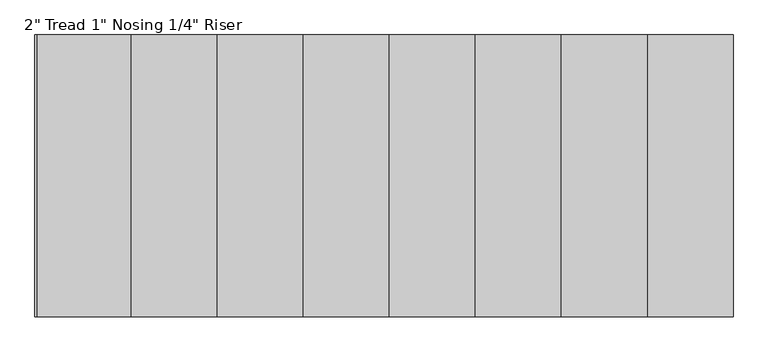
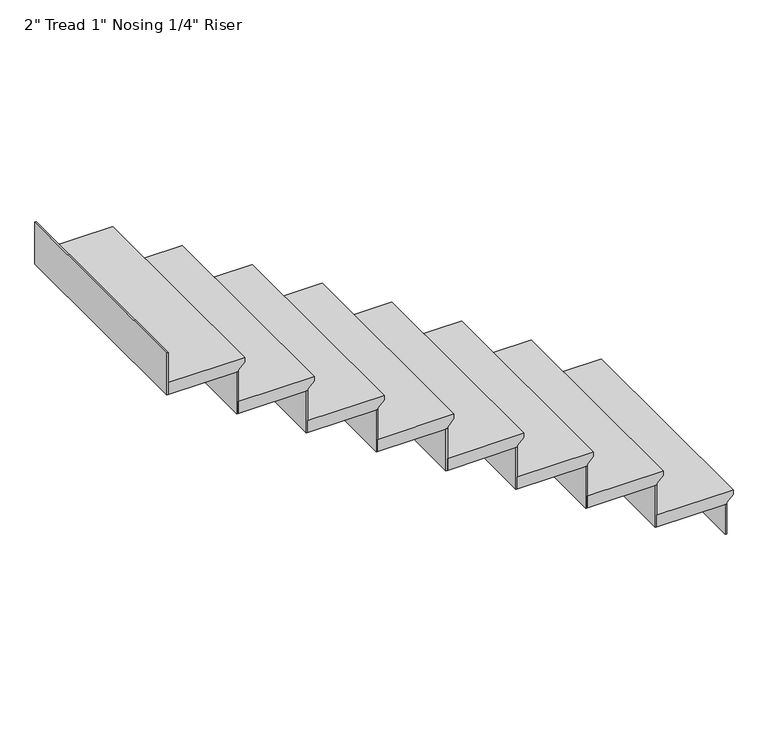
"""IFC4 building model written with IfcOpenShell, lengths in millimetres: stair flight geometry."""

from ifc_helpers import new_model, si_unit, origin, place, context, project, spatial, faceted_brep, source, transform, mapped, element, save


def stair_flight_1f3fe34f(model_context):
    return source(origin(), model_context, "Body", "Brep", [
        faceted_brep([(-3245.3112714, -4870.057676, 6559.55), (-3245.3112714, -4870.057676, 6578.6), (-3245.3112714, -5784.457676, 6578.6), (-3245.3112714, -5784.457676, 6559.55), (-3270.7112714, -4870.057676, 6534.15), (-3270.7112714, -5784.457676, 6534.15), (-3550.1112714, -4870.057676, 6578.6), (-3550.1112714, -5784.457676, 6578.6), (-3270.7112714, -5784.457676, 6527.8), (-3550.1112714, -5784.457676, 6527.8), (-3550.1112714, -4870.057676, 6527.8), (-3270.7112714, -4870.057676, 6527.8)], [[[0, 1, 2, 3]], [[4, 0, 3, 5]], [[2, 1, 6, 7]], [[8, 9, 10, 11]], [[2, 7, 9, 8, 5, 3]], [[8, 11, 4, 5]], [[6, 1, 0, 4, 11, 10]], [[7, 6, 10, 9]]]),
        faceted_brep([(-3270.7112714, -4870.057676, 6527.8), (-3270.7112714, -4870.057676, 6400.8), (-3277.0612714, -4870.057676, 6400.8), (-3277.0612714, -4870.057676, 6527.8), (-3270.7112714, -5784.457676, 6527.8), (-3277.0612714, -5784.457676, 6527.8), (-3277.0612714, -5784.457676, 6400.8), (-3270.7112714, -5784.457676, 6400.8)], [[[0, 1, 2, 3]], [[4, 5, 6, 7]], [[1, 0, 4, 7]], [[2, 1, 7, 6]], [[3, 2, 6, 5]], [[0, 3, 5, 4]]]),
        faceted_brep([(-5505.9112714, -4870.057676, 7950.2), (-5505.9112714, -4870.057676, 7772.4), (-5512.2612714, -4870.057676, 7772.4), (-5512.2612714, -4870.057676, 7950.2), (-5505.9112714, -5784.457676, 7950.2), (-5512.2612714, -5784.457676, 7950.2), (-5512.2612714, -5784.457676, 7772.4), (-5505.9112714, -5784.457676, 7772.4)], [[[0, 1, 2, 3]], [[4, 5, 6, 7]], [[1, 0, 4, 7]], [[2, 1, 7, 6]], [[3, 2, 6, 5]], [[0, 3, 5, 4]]]),
        faceted_brep([(-3550.1112714, -4870.057676, 6705.6), (-3550.1112714, -4870.057676, 6527.8), (-3556.4612714, -4870.057676, 6527.8), (-3556.4612714, -4870.057676, 6705.6), (-3550.1112714, -5784.457676, 6705.6), (-3556.4612714, -5784.457676, 6705.6), (-3556.4612714, -5784.457676, 6527.8), (-3550.1112714, -5784.457676, 6527.8)], [[[0, 1, 2, 3]], [[4, 5, 6, 7]], [[1, 0, 4, 7]], [[2, 1, 7, 6]], [[3, 2, 6, 5]], [[0, 3, 5, 4]]]),
        faceted_brep([(-3524.7112714, -5784.457676, 6756.4), (-3524.7112714, -4870.057676, 6756.4), (-3829.5112714, -4870.057676, 6756.4), (-3829.5112714, -5784.457676, 6756.4), (-3550.1112714, -5784.457676, 6705.6), (-3829.5112714, -5784.457676, 6705.6), (-3829.5112714, -4870.057676, 6705.6), (-3550.1112714, -4870.057676, 6705.6), (-3550.1112714, -5784.457676, 6711.95), (-3524.7112714, -5784.457676, 6737.35), (-3550.1112714, -4870.057676, 6711.95), (-3524.7112714, -4870.057676, 6737.35)], [[[0, 1, 2, 3]], [[4, 5, 6, 7]], [[0, 3, 5, 4, 8, 9]], [[4, 7, 10, 8]], [[2, 1, 11, 10, 7, 6]], [[3, 2, 6, 5]], [[11, 1, 0, 9]], [[10, 11, 9, 8]]]),
        faceted_brep([(-3829.5112714, -4870.057676, 6883.4), (-3829.5112714, -4870.057676, 6705.6), (-3835.8612714, -4870.057676, 6705.6), (-3835.8612714, -4870.057676, 6883.4), (-3829.5112714, -5784.457676, 6883.4), (-3835.8612714, -5784.457676, 6883.4), (-3835.8612714, -5784.457676, 6705.6), (-3829.5112714, -5784.457676, 6705.6)], [[[0, 1, 2, 3]], [[4, 5, 6, 7]], [[1, 0, 4, 7]], [[2, 1, 7, 6]], [[3, 2, 6, 5]], [[0, 3, 5, 4]]]),
        faceted_brep([(-3804.1112714, -5784.457676, 6934.2), (-3804.1112714, -4870.057676, 6934.2), (-4108.9112714, -4870.057676, 6934.2), (-4108.9112714, -5784.457676, 6934.2), (-3829.5112714, -5784.457676, 6883.4), (-4108.9112714, -5784.457676, 6883.4), (-4108.9112714, -4870.057676, 6883.4), (-3829.5112714, -4870.057676, 6883.4), (-3829.5112714, -5784.457676, 6889.75), (-3804.1112714, -5784.457676, 6915.15), (-3829.5112714, -4870.057676, 6889.75), (-3804.1112714, -4870.057676, 6915.15)], [[[0, 1, 2, 3]], [[4, 5, 6, 7]], [[0, 3, 5, 4, 8, 9]], [[4, 7, 10, 8]], [[2, 1, 11, 10, 7, 6]], [[3, 2, 6, 5]], [[11, 1, 0, 9]], [[10, 11, 9, 8]]]),
        faceted_brep([(-4108.9112714, -4870.057676, 7061.2), (-4108.9112714, -4870.057676, 6883.4), (-4115.2612714, -4870.057676, 6883.4), (-4115.2612714, -4870.057676, 7061.2), (-4108.9112714, -5784.457676, 7061.2), (-4115.2612714, -5784.457676, 7061.2), (-4115.2612714, -5784.457676, 6883.4), (-4108.9112714, -5784.457676, 6883.4)], [[[0, 1, 2, 3]], [[4, 5, 6, 7]], [[1, 0, 4, 7]], [[2, 1, 7, 6]], [[3, 2, 6, 5]], [[0, 3, 5, 4]]]),
        faceted_brep([(-4083.5112714, -5784.457676, 7112.0), (-4083.5112714, -4870.057676, 7112.0), (-4388.3112714, -4870.057676, 7112.0), (-4388.3112714, -5784.457676, 7112.0), (-4108.9112714, -5784.457676, 7061.2), (-4388.3112714, -5784.457676, 7061.2), (-4388.3112714, -4870.057676, 7061.2), (-4108.9112714, -4870.057676, 7061.2), (-4108.9112714, -5784.457676, 7067.55), (-4083.5112714, -5784.457676, 7092.95), (-4108.9112714, -4870.057676, 7067.55), (-4083.5112714, -4870.057676, 7092.95)], [[[0, 1, 2, 3]], [[4, 5, 6, 7]], [[0, 3, 5, 4, 8, 9]], [[4, 7, 10, 8]], [[2, 1, 11, 10, 7, 6]], [[3, 2, 6, 5]], [[11, 1, 0, 9]], [[10, 11, 9, 8]]]),
        faceted_brep([(-4388.3112714, -4870.057676, 7239.0), (-4388.3112714, -4870.057676, 7061.2), (-4394.6612714, -4870.057676, 7061.2), (-4394.6612714, -4870.057676, 7239.0), (-4388.3112714, -5784.457676, 7239.0), (-4394.6612714, -5784.457676, 7239.0), (-4394.6612714, -5784.457676, 7061.2), (-4388.3112714, -5784.457676, 7061.2)], [[[0, 1, 2, 3]], [[4, 5, 6, 7]], [[1, 0, 4, 7]], [[2, 1, 7, 6]], [[3, 2, 6, 5]], [[0, 3, 5, 4]]]),
        faceted_brep([(-4362.9112714, -5784.457676, 7289.8), (-4362.9112714, -4870.057676, 7289.8), (-4667.7112714, -4870.057676, 7289.8), (-4667.7112714, -5784.457676, 7289.8), (-4388.3112714, -5784.457676, 7239.0), (-4667.7112714, -5784.457676, 7239.0), (-4667.7112714, -4870.057676, 7239.0), (-4388.3112714, -4870.057676, 7239.0), (-4388.3112714, -5784.457676, 7245.35), (-4362.9112714, -5784.457676, 7270.75), (-4388.3112714, -4870.057676, 7245.35), (-4362.9112714, -4870.057676, 7270.75)], [[[0, 1, 2, 3]], [[4, 5, 6, 7]], [[0, 3, 5, 4, 8, 9]], [[4, 7, 10, 8]], [[2, 1, 11, 10, 7, 6]], [[3, 2, 6, 5]], [[11, 1, 0, 9]], [[10, 11, 9, 8]]]),
        faceted_brep([(-4667.7112714, -4870.057676, 7416.8), (-4667.7112714, -4870.057676, 7239.0), (-4674.0612714, -4870.057676, 7239.0), (-4674.0612714, -4870.057676, 7416.8), (-4667.7112714, -5784.457676, 7416.8), (-4674.0612714, -5784.457676, 7416.8), (-4674.0612714, -5784.457676, 7239.0), (-4667.7112714, -5784.457676, 7239.0)], [[[0, 1, 2, 3]], [[4, 5, 6, 7]], [[1, 0, 4, 7]], [[2, 1, 7, 6]], [[3, 2, 6, 5]], [[0, 3, 5, 4]]]),
        faceted_brep([(-4642.3112714, -5784.457676, 7467.6), (-4642.3112714, -4870.057676, 7467.6), (-4947.1112714, -4870.057676, 7467.6), (-4947.1112714, -5784.457676, 7467.6), (-4667.7112714, -5784.457676, 7416.8), (-4947.1112714, -5784.457676, 7416.8), (-4947.1112714, -4870.057676, 7416.8), (-4667.7112714, -4870.057676, 7416.8), (-4667.7112714, -5784.457676, 7423.15), (-4642.3112714, -5784.457676, 7448.55), (-4667.7112714, -4870.057676, 7423.15), (-4642.3112714, -4870.057676, 7448.55)], [[[0, 1, 2, 3]], [[4, 5, 6, 7]], [[0, 3, 5, 4, 8, 9]], [[4, 7, 10, 8]], [[2, 1, 11, 10, 7, 6]], [[3, 2, 6, 5]], [[11, 1, 0, 9]], [[10, 11, 9, 8]]]),
        faceted_brep([(-4947.1112714, -4870.057676, 7594.6), (-4947.1112714, -4870.057676, 7416.8), (-4953.4612714, -4870.057676, 7416.8), (-4953.4612714, -4870.057676, 7594.6), (-4947.1112714, -5784.457676, 7594.6), (-4953.4612714, -5784.457676, 7594.6), (-4953.4612714, -5784.457676, 7416.8), (-4947.1112714, -5784.457676, 7416.8)], [[[0, 1, 2, 3]], [[4, 5, 6, 7]], [[1, 0, 4, 7]], [[2, 1, 7, 6]], [[3, 2, 6, 5]], [[0, 3, 5, 4]]]),
        faceted_brep([(-4921.7112714, -5784.457676, 7645.4), (-4921.7112714, -4870.057676, 7645.4), (-5226.5112714, -4870.057676, 7645.4), (-5226.5112714, -5784.457676, 7645.4), (-4947.1112714, -5784.457676, 7594.6), (-5226.5112714, -5784.457676, 7594.6), (-5226.5112714, -4870.057676, 7594.6), (-4947.1112714, -4870.057676, 7594.6), (-4947.1112714, -5784.457676, 7600.95), (-4921.7112714, -5784.457676, 7626.35), (-4947.1112714, -4870.057676, 7600.95), (-4921.7112714, -4870.057676, 7626.35)], [[[0, 1, 2, 3]], [[4, 5, 6, 7]], [[0, 3, 5, 4, 8, 9]], [[4, 7, 10, 8]], [[2, 1, 11, 10, 7, 6]], [[3, 2, 6, 5]], [[11, 1, 0, 9]], [[10, 11, 9, 8]]]),
        faceted_brep([(-5226.5112714, -4870.057676, 7772.4), (-5226.5112714, -4870.057676, 7594.6), (-5232.8612714, -4870.057676, 7594.6), (-5232.8612714, -4870.057676, 7772.4), (-5226.5112714, -5784.457676, 7772.4), (-5232.8612714, -5784.457676, 7772.4), (-5232.8612714, -5784.457676, 7594.6), (-5226.5112714, -5784.457676, 7594.6)], [[[0, 1, 2, 3]], [[4, 5, 6, 7]], [[1, 0, 4, 7]], [[2, 1, 7, 6]], [[3, 2, 6, 5]], [[0, 3, 5, 4]]]),
        faceted_brep([(-5201.1112714, -5784.457676, 7823.2), (-5201.1112714, -4870.057676, 7823.2), (-5480.5112714, -4870.057676, 7823.2), (-5505.9112714, -4870.057676, 7823.2), (-5505.9112714, -5784.457676, 7823.2), (-5226.5112714, -5784.457676, 7772.4), (-5505.9112714, -5784.457676, 7772.4), (-5505.9112714, -4870.057676, 7772.4), (-5480.5112714, -4870.057676, 7772.4), (-5226.5112714, -4870.057676, 7772.4), (-5226.5112714, -5784.457676, 7778.75), (-5201.1112714, -5784.457676, 7804.15), (-5226.5112714, -4870.057676, 7778.75), (-5201.1112714, -4870.057676, 7804.15)], [[[0, 1, 2, 3, 4]], [[5, 6, 7, 8, 9]], [[0, 4, 6, 5, 10, 11]], [[5, 9, 12, 10]], [[2, 1, 13, 12, 9, 8]], [[3, 2, 8, 7]], [[4, 3, 7, 6]], [[13, 1, 0, 11]], [[12, 13, 11, 10]]]),
    ])


if __name__ == "__main__":
    model = new_model("IFC4")
    model_context = context("Model", 3, world=origin())
    ifc_project = project(units=[si_unit("LENGTHUNIT", "METRE", prefix="MILLI")], contexts=[model_context])
    site = spatial("IfcSite", under=ifc_project)
    building = spatial("IfcBuilding", under=site)
    placement = place(None, origin())
    stair_flight_shape = stair_flight_1f3fe34f(model_context)
    element("IfcStairFlight", 1, ObjectType="2\" Tread 1\" Nosing 1/4\" Riser", at=placement, inside=building, context=model_context, shape_type="MappedRepresentation", body=[
        mapped(stair_flight_shape, transform((0.0, 0.0, 0.0), x_axis=(1.0, 0.0, 0.0), y_axis=(0.0, 1.0, 0.0), z_axis=(0.0, 0.0, 1.0))),
    ])
    save(model, "model.ifc")
